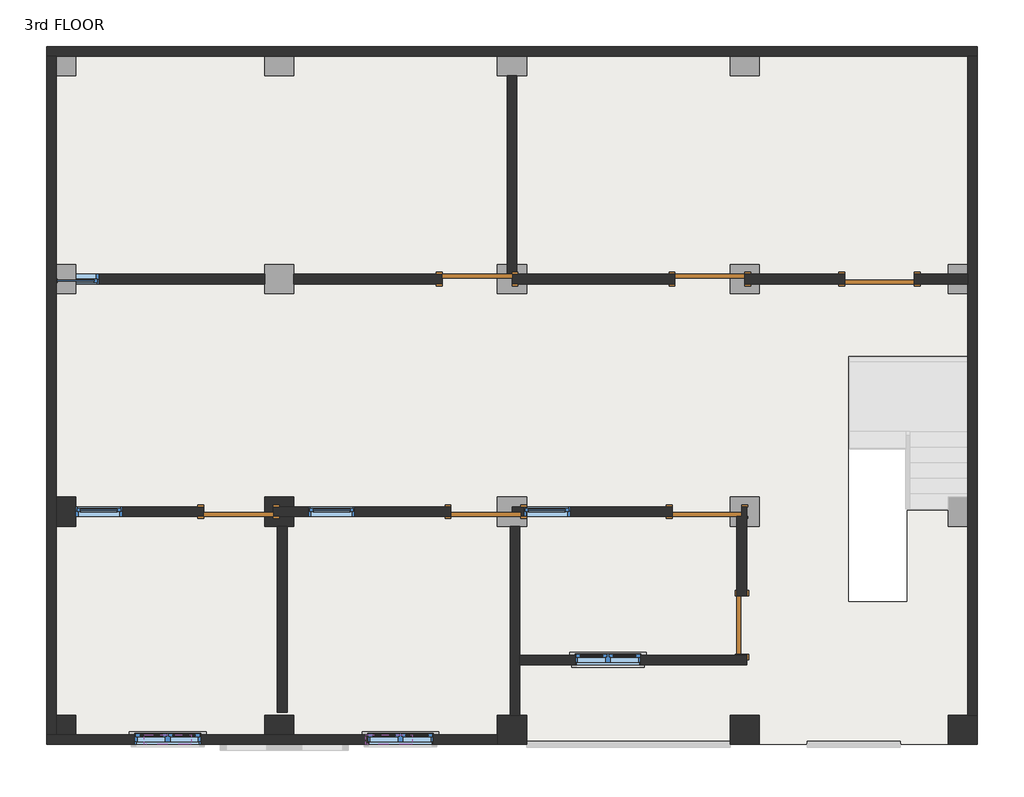
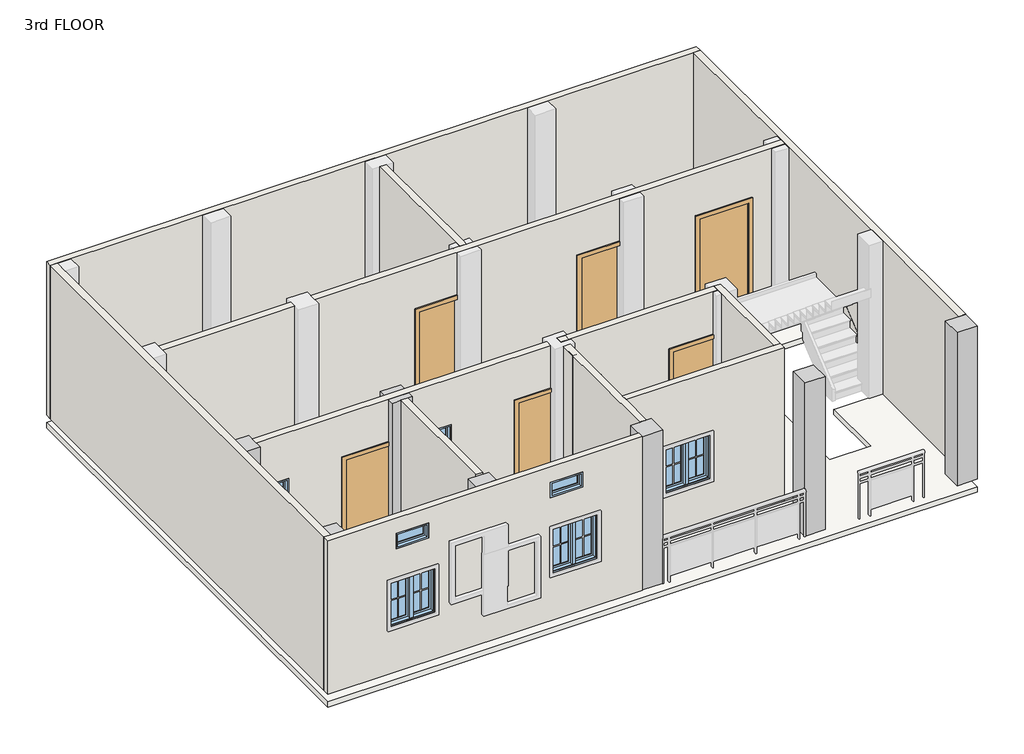
# One storey, part 1 of 2: 15 walls, 9 windows, 7 columns, 7 doors, 1 slab.
"""IFC4 building model written with IfcOpenShell, lengths in millimetres."""

from ifc_helpers import new_model, si_unit, frame, origin, place, context, project, spatial, polyline, outline, extrude, faceted_brep, transform, mapped, element, save
from components import door_e00f436c, door_a1797ceb, window_4c2727af, window_0bf3737e, window_78893e6c, window_0d9958e7

model = new_model("IFC4")

# Units and contexts
model_context = context("Model", 3, world=origin())
ifc_project = project(units=[si_unit("LENGTHUNIT", "METRE", prefix="MILLI")], contexts=[model_context])

# Site, building, storey
site = spatial("IfcSite", under=ifc_project)
building = spatial("IfcBuilding", under=site)
storey = spatial("IfcBuildingStorey", under=building, Name="3rd FLOOR", Elevation=8991.6)

# Columns
placement = place(None, origin())
element("IfcColumn", 1, ObjectType="column family : column family", at=placement, inside=storey, context=model_context, shape_type="Brep", body=[
    faceted_brep([(-12576.097125, 2486.2065522, 8996.6), (-12957.097125, 2486.2065522, 8996.6), (-12957.097125, 2867.2065522, 8996.6), (-12576.097125, 2867.2065522, 8996.6), (-12576.097125, 2740.2065522, 8996.6), (-12842.797125, 2740.2065522, 8996.6), (-12842.797125, 2613.2065522, 8996.6), (-12576.097125, 2613.2065522, 8996.6), (-12576.097125, 2486.2065522, 12034.6), (-12576.097125, 2613.2065522, 12034.6), (-12957.097125, 2486.2065522, 12034.6), (-12957.097125, 2613.2065522, 12034.6), (-12957.097125, 2613.2065522, 11125.2), (-12957.097125, 2740.2065522, 11125.2), (-12957.097125, 2740.2065522, 12034.6), (-12957.097125, 2867.2065522, 12034.6), (-12576.097125, 2867.2065522, 12034.6), (-12842.797125, 2613.2065522, 11125.2), (-12842.797125, 2740.2065522, 11125.2), (-12576.097125, 2740.2065522, 12034.6)], [[[0, 1, 2, 3, 4, 5, 6, 7]], [[8, 0, 7, 9]], [[1, 0, 8, 10]], [[2, 1, 10, 11, 12, 13, 14, 15]], [[3, 2, 15, 16]], [[10, 8, 9, 11]], [[6, 17, 12, 11, 9, 7]], [[13, 18, 5, 4, 19, 14]], [[3, 16, 19, 4]], [[16, 15, 14, 19]], [[17, 18, 13, 12]], [[18, 17, 6, 5]]]),
])
element("IfcColumn", 2, ObjectType="column family : column family", at=placement, inside=storey, context=model_context, shape_type="SweptSolid", body=[
    extrude(outline(polyline([(-15433.597125, 2867.2065522), (-15433.597125, 2486.2065522), (-15687.597125, 2486.2065522), (-15687.597125, 2867.2065522), (-15433.597125, 2867.2065522)])), frame((0.0, 0.0, 8996.6), z_axis=(0.0, 0.0, 1.0), x_axis=(1.0, 0.0, 0.0)), (0.0, 0.0, 1.0), 3038.0),
])
element("IfcColumn", 3, ObjectType="column family : column family", at=placement, inside=storey, context=model_context, shape_type="SweptSolid", body=[
    extrude(outline(polyline([(-15433.597125, 9.7065522), (-15433.597125, -244.2934478), (-15687.597125, -244.2934478), (-15687.597125, 9.7065522), (-15433.597125, 9.7065522)])), frame((0.0, 0.0, 8996.6), z_axis=(0.0, 0.0, 1.0), x_axis=(1.0, 0.0, 0.0)), (0.0, 0.0, 1.0), 3038.0),
])
element("IfcColumn", 4, ObjectType="column family : column family", at=placement, inside=storey, context=model_context, shape_type="SweptSolid", body=[
    extrude(outline(polyline([(-3622.597125, 9.7065522), (-3622.597125, -371.2934478), (-4003.597125, -371.2934478), (-4003.597125, 9.7065522), (-3622.597125, 9.7065522)])), frame((0.0, 0.0, 8996.6), z_axis=(0.0, 0.0, 1.0), x_axis=(1.0, 0.0, 0.0)), (0.0, 0.0, 1.0), 3038.0),
])
element("IfcColumn", 5, ObjectType="column family : column family", at=placement, inside=storey, context=model_context, shape_type="SweptSolid", body=[
    extrude(outline(polyline([(-6480.097125, 9.7065522), (-6480.097125, -371.2934478), (-6861.097125, -371.2934478), (-6861.097125, 9.7065522), (-6480.097125, 9.7065522)])), frame((0.0, 0.0, 8996.6), z_axis=(0.0, 0.0, 1.0), x_axis=(1.0, 0.0, 0.0)), (0.0, 0.0, 1.0), 3038.0),
])
element("IfcColumn", 6, ObjectType="column family : column family", at=placement, inside=storey, context=model_context, shape_type="SweptSolid", body=[
    extrude(outline(polyline([(-9528.097125, 9.7065522), (-9528.097125, -371.2934478), (-9909.097125, -371.2934478), (-9909.097125, 9.7065522), (-9528.097125, 9.7065522)])), frame((0.0, 0.0, 8996.6), z_axis=(0.0, 0.0, 1.0), x_axis=(1.0, 0.0, 0.0)), (0.0, 0.0, 1.0), 3038.0),
])
element("IfcColumn", 7, ObjectType="column family : column family", at=placement, inside=storey, context=model_context, shape_type="SweptSolid", body=[
    extrude(outline(polyline([(-12957.097125, 9.7065522), (-12576.097125, 9.7065522), (-12576.097125, -244.2934478), (-12957.097125, -244.2934478), (-12957.097125, 9.7065522)])), frame((0.0, 0.0, 8996.6), z_axis=(0.0, 0.0, 1.0), x_axis=(1.0, 0.0, 0.0)), (0.0, 0.0, 1.0), 3038.0),
])

# Doors
door_shape = door_e00f436c(model_context)
element("IfcDoor", 8, ObjectType="Single-Flush : 30\" x 80\"", at=placement, inside=storey, context=model_context, shape_type="MappedRepresentation", body=[
    mapped(door_shape, transform((-6708.697125, 1190.8065522, 8991.6), x_axis=(0.0, -1.0, 0.0), y_axis=(1.0, 0.0, 0.0), z_axis=(0.0, 0.0, 1.0))),
])
door_2_shape = door_a1797ceb(model_context)
element("IfcDoor", 9, ObjectType="Single-Flush : 36\" x 84\"", at=placement, inside=storey, context=model_context, shape_type="MappedRepresentation", body=[
    mapped(door_2_shape, transform((-10175.797125, 5724.7065522, 8991.6), x_axis=(1.0, 0.0, 0.0), y_axis=(0.0, 1.0, 0.0), z_axis=(0.0, 0.0, 1.0))),
])
element("IfcDoor", 10, ObjectType="Single-Flush : 36\" x 84\"", at=placement, inside=storey, context=model_context, shape_type="MappedRepresentation", body=[
    mapped(door_2_shape, transform((-10061.497125, 2676.7065522, 8991.6), x_axis=(-1.0, 0.0, 0.0), y_axis=(0.0, -1.0, 0.0), z_axis=(0.0, 0.0, 1.0))),
])
element("IfcDoor", 11, ObjectType="Single-Flush : 36\" x 84\"", at=placement, inside=storey, context=model_context, shape_type="MappedRepresentation", body=[
    mapped(door_2_shape, transform((-13299.997125, 2676.7065522, 8991.6), x_axis=(-1.0, 0.0, 0.0), y_axis=(0.0, -1.0, 0.0), z_axis=(0.0, 0.0, 1.0))),
])
element("IfcDoor", 12, ObjectType="Single-Flush : 36\" x 84\"", at=placement, inside=storey, context=model_context, shape_type="MappedRepresentation", body=[
    mapped(door_2_shape, transform((-7127.797125, 5724.7065522, 8991.6), x_axis=(1.0, 0.0, 0.0), y_axis=(0.0, 1.0, 0.0), z_axis=(0.0, 0.0, 1.0))),
])
element("IfcDoor", 13, ObjectType="Single-Flush : 36\" x 84\"", at=placement, inside=storey, context=model_context, shape_type="MappedRepresentation", body=[
    mapped(door_2_shape, transform((-7165.897125, 2676.7065522, 8991.6), x_axis=(-1.0, 0.0, 0.0), y_axis=(0.0, -1.0, 0.0), z_axis=(0.0, 0.0, 1.0))),
])
element("IfcDoor", 14, ObjectType="Single-Flush : 36\" x 84\"", at=placement, inside=storey, context=model_context, shape_type="MappedRepresentation", body=[
    mapped(door_2_shape, transform((-4905.297125, 5724.7065522, 8991.6), x_axis=(-1.0, 0.0, 0.0), y_axis=(0.0, -1.0, 0.0), z_axis=(0.0, 0.0, 1.0))),
])

# Slab
element("IfcSlab", 15, ObjectType="Generic - 4\"", at=placement, inside=storey, context=model_context, shape_type="SweptSolid", body=[
    extrude(outline(polyline([(-3622.597125, 8772.7065522), (-3622.597125, -371.2934478), (-15814.597125, -371.2934478), (-15814.597125, 8772.7065522), (-3622.597125, 8772.7065522)]), holes=[polyline([(-3734.357125, 4711.0719226), (-5310.2646464, 4711.0719226), (-5310.2646464, 1502.3126957), (-4547.7736682, 1502.3126957), (-4547.7736682, 2699.911213), (-3734.357125, 2699.911213), (-3734.357125, 4711.0719226)])]), frame((0.0, 0.0, 8737.6), z_axis=(0.0, 0.0, 1.0), x_axis=(1.0, 0.0, 0.0)), (0.0, 0.0, 1.0), 101.6),
])

# Walls
element("IfcWall", 16, ObjectType="Generic - 5\"", at=placement, inside=storey, context=model_context, shape_type="Brep", body=[
    faceted_brep([(-15814.597125, 8645.7065522, 8991.6), (-15687.597125, 8645.7065522, 8991.6), (-3749.597125, 8645.7065522, 8991.6), (-3622.597125, 8645.7065522, 8991.6), (-3622.597125, 8645.7065522, 12039.6), (-3749.597125, 8645.7065522, 12039.6), (-15687.597125, 8645.7065522, 12039.6), (-15814.597125, 8645.7065522, 12039.6), (-15814.597125, 8772.7065522, 8991.6), (-15814.597125, 8772.7065522, 12039.6), (-3622.597125, 8772.7065522, 12039.6), (-3622.597125, 8772.7065522, 8991.6)], [[[0, 1, 2, 3, 4, 5, 6, 7]], [[8, 9, 10, 11]], [[3, 2, 1, 0, 8, 11]], [[7, 6, 5, 4, 10, 9]], [[4, 3, 11, 10]], [[0, 7, 9, 8]]]),
])
element("IfcWall", 17, ObjectType="Generic - 5\"", at=placement, inside=storey, context=model_context, shape_type="Brep", body=[
    faceted_brep([(-3749.597125, 8645.7065522, 8991.6), (-3749.597125, 5788.2065522, 8991.6), (-3749.597125, 5661.2065522, 8991.6), (-3749.597125, 9.7065522, 8991.6), (-3749.597125, 9.7065522, 12039.6), (-3749.597125, 5661.2065522, 12039.6), (-3749.597125, 5788.2065522, 12039.6), (-3749.597125, 8645.7065522, 12039.6), (-3622.597125, 8645.7065522, 8991.6), (-3622.597125, 8645.7065522, 12039.6), (-3622.597125, 9.7065522, 12039.6), (-3622.597125, 9.7065522, 12034.6), (-3622.597125, 9.7065522, 8996.6), (-3622.597125, 9.7065522, 8991.6)], [[[0, 1, 2, 3, 4, 5, 6, 7]], [[8, 9, 10, 11, 12, 13]], [[3, 2, 1, 0, 8, 13]], [[4, 3, 13, 12, 11, 10]], [[7, 6, 5, 4, 10, 9]], [[0, 7, 9, 8]]]),
])
element("IfcWall", 18, ObjectType="Generic - 5\"", at=placement, inside=storey, context=model_context, shape_type="Brep", body=[
    faceted_brep([(-9909.097125, -244.2934478, 8991.6), (-15687.597125, -244.2934478, 8991.6), (-15814.597125, -244.2934478, 8991.6), (-15814.597125, -244.2934478, 12039.6), (-15687.597125, -244.2934478, 12039.6), (-9909.097125, -244.2934478, 12039.6), (-13795.297125, -244.2934478, 10820.4), (-14658.897125, -244.2934478, 10820.4), (-14658.897125, -244.2934478, 9906.0), (-13795.297125, -244.2934478, 9906.0), (-10747.297125, -244.2934478, 10820.4), (-11610.897125, -244.2934478, 10820.4), (-11610.897125, -244.2934478, 9906.0), (-10747.297125, -244.2934478, 9906.0), (-13922.297125, -244.2934478, 11734.8), (-14531.897125, -244.2934478, 11734.8), (-14531.897125, -244.2934478, 11430.0), (-13922.297125, -244.2934478, 11430.0), (-11026.697125, -244.2934478, 11734.8), (-11636.297125, -244.2934478, 11734.8), (-11636.297125, -244.2934478, 11430.0), (-11026.697125, -244.2934478, 11430.0), (-9909.097125, -371.2934478, 8991.6), (-9909.097125, -371.2934478, 8996.6), (-9909.097125, -371.2934478, 12034.6), (-9909.097125, -371.2934478, 12039.6), (-15814.597125, -371.2934478, 12039.6), (-15814.597125, -371.2934478, 8991.6), (-13795.297125, -371.2934478, 10820.4), (-13795.297125, -371.2934478, 9906.0), (-14658.897125, -371.2934478, 9906.0), (-14658.897125, -371.2934478, 10820.4), (-10747.297125, -371.2934478, 10820.4), (-10747.297125, -371.2934478, 9906.0), (-11610.897125, -371.2934478, 9906.0), (-11610.897125, -371.2934478, 10820.4), (-13922.297125, -371.2934478, 11734.8), (-13922.297125, -371.2934478, 11430.0), (-14531.897125, -371.2934478, 11430.0), (-14531.897125, -371.2934478, 11734.8), (-11026.697125, -371.2934478, 11734.8), (-11026.697125, -371.2934478, 11430.0), (-11636.297125, -371.2934478, 11430.0), (-11636.297125, -371.2934478, 11734.8)], [[[0, 1, 2, 3, 4, 5], [6, 7, 8, 9], [10, 11, 12, 13], [14, 15, 16, 17], [18, 19, 20, 21]], [[22, 23, 24, 25, 26, 27], [28, 29, 30, 31], [32, 33, 34, 35], [36, 37, 38, 39], [40, 41, 42, 43]], [[2, 1, 0, 22, 27]], [[5, 4, 3, 26, 25]], [[0, 5, 25, 24, 23, 22]], [[3, 2, 27, 26]], [[29, 28, 6, 9]], [[30, 29, 9, 8]], [[31, 30, 8, 7]], [[28, 31, 7, 6]], [[33, 32, 10, 13]], [[34, 33, 13, 12]], [[35, 34, 12, 11]], [[32, 35, 11, 10]], [[37, 36, 14, 17]], [[38, 37, 17, 16]], [[39, 38, 16, 15]], [[36, 39, 15, 14]], [[41, 40, 18, 21]], [[42, 41, 21, 20]], [[43, 42, 20, 19]], [[40, 43, 19, 18]]]),
])
element("IfcWall", 19, ObjectType="Generic - 5\"", at=placement, inside=storey, context=model_context, shape_type="Brep", body=[
    faceted_brep([(-15687.597125, -244.2934478, 8991.6), (-15687.597125, 8645.7065522, 8991.6), (-15687.597125, 8645.7065522, 8996.6), (-15687.597125, 8645.7065522, 12034.6), (-15687.597125, 8645.7065522, 12039.6), (-15687.597125, -244.2934478, 12039.6), (-15687.597125, -244.2934478, 12034.6), (-15687.597125, -244.2934478, 8996.6), (-15814.597125, -244.2934478, 8991.6), (-15814.597125, -244.2934478, 12039.6), (-15814.597125, 8645.7065522, 12039.6), (-15814.597125, 8645.7065522, 8991.6)], [[[0, 1, 2, 3, 4, 5, 6, 7]], [[8, 9, 10, 11]], [[1, 0, 8, 11]], [[5, 4, 10, 9]], [[4, 3, 2, 1, 11, 10]], [[0, 7, 6, 5, 9, 8]]]),
])
element("IfcWall", 20, ObjectType="Generic - 5\"", at=placement, inside=storey, context=model_context, shape_type="SweptSolid", body=[
    extrude(outline(polyline([(8991.6, -15433.597125), (8991.6, -12957.097125), (12039.6, -12957.097125), (12039.6, -15433.597125), (11125.2, -15433.597125), (11125.2, -15128.797125), (9296.4, -15128.797125), (9296.4, -15433.597125), (8991.6, -15433.597125)])), frame((0.0, 5661.2065522, 0.0), z_axis=(0.0, 1.0, 0.0), x_axis=(0.0, 0.0, 1.0)), (0.0, 0.0, 1.0), 127.0),
])
element("IfcWall", 21, ObjectType="Generic - 5\"", at=placement, inside=storey, context=model_context, shape_type="Brep", body=[
    faceted_brep([(-9782.097125, 8391.7065522, 8991.6), (-9782.097125, 5788.2065522, 8991.6), (-9782.097125, 5788.2065522, 8996.6), (-9782.097125, 5788.2065522, 11125.2), (-9782.097125, 5788.2065522, 12034.6), (-9782.097125, 5788.2065522, 12039.6), (-9782.097125, 8391.7065522, 12039.6), (-9655.097125, 8391.7065522, 8991.6), (-9655.097125, 8391.7065522, 12039.6), (-9655.097125, 5788.2065522, 12039.6), (-9655.097125, 5788.2065522, 12034.6), (-9655.097125, 5788.2065522, 8996.6), (-9655.097125, 5788.2065522, 8991.6), (-9718.597125, 5788.2065522, 8991.6)], [[[0, 1, 2, 3, 4, 5, 6]], [[7, 8, 9, 10, 11, 12]], [[1, 0, 7, 12, 13]], [[6, 5, 9, 8]], [[0, 6, 8, 7]], [[5, 4, 3, 2, 1, 13, 12, 11, 10, 9]]]),
])
element("IfcWall", 22, ObjectType="Generic - 5\"", at=placement, inside=storey, context=model_context, shape_type="Brep", body=[
    faceted_brep([(-6670.597125, 5661.2065522, 8991.6), (-5362.497125, 5661.2065522, 8991.6), (-5362.497125, 5661.2065522, 11125.2), (-4448.097125, 5661.2065522, 11125.2), (-4448.097125, 5661.2065522, 8991.6), (-3749.597125, 5661.2065522, 8991.6), (-3749.597125, 5661.2065522, 8996.6), (-3749.597125, 5661.2065522, 12034.6), (-3749.597125, 5661.2065522, 12039.6), (-12576.097125, 5661.2065522, 12039.6), (-12576.097125, 5661.2065522, 8991.6), (-10632.997125, 5661.2065522, 8991.6), (-10632.997125, 5661.2065522, 11125.2), (-9909.097125, 5661.2065522, 11125.2), (-9718.597125, 5661.2065522, 11125.2), (-9718.597125, 5661.2065522, 8996.6), (-9718.597125, 5661.2065522, 8991.6), (-7584.997125, 5661.2065522, 8991.6), (-7584.997125, 5661.2065522, 11125.2), (-6861.097125, 5661.2065522, 11125.2), (-6670.597125, 5661.2065522, 11125.2), (-6670.597125, 5661.2065522, 8996.6), (-5362.497125, 5788.2065522, 11125.2), (-5362.497125, 5788.2065522, 8991.6), (-6670.597125, 5788.2065522, 8991.6), (-6670.597125, 5788.2065522, 8996.6), (-6670.597125, 5788.2065522, 11125.2), (-6861.097125, 5788.2065522, 11125.2), (-7584.997125, 5788.2065522, 11125.2), (-7584.997125, 5788.2065522, 8991.6), (-9655.097125, 5788.2065522, 8991.6), (-9718.597125, 5788.2065522, 8991.6), (-9718.597125, 5788.2065522, 8996.6), (-9718.597125, 5788.2065522, 11125.2), (-9782.097125, 5788.2065522, 11125.2), (-9909.097125, 5788.2065522, 11125.2), (-10632.997125, 5788.2065522, 11125.2), (-10632.997125, 5788.2065522, 8991.6), (-12576.097125, 5788.2065522, 8991.6), (-12576.097125, 5788.2065522, 12039.6), (-9782.097125, 5788.2065522, 12039.6), (-9655.097125, 5788.2065522, 12039.6), (-3749.597125, 5788.2065522, 12039.6), (-3749.597125, 5788.2065522, 12034.6), (-3749.597125, 5788.2065522, 8996.6), (-3749.597125, 5788.2065522, 8991.6), (-4448.097125, 5788.2065522, 8991.6), (-4448.097125, 5788.2065522, 11125.2)], [[[0, 1, 2, 3, 4, 5, 6, 7, 8, 9, 10, 11, 12, 13, 14, 15, 16, 17, 18, 19, 20, 21]], [[22, 23, 24, 25, 26, 27, 28, 29, 30, 31, 32, 33, 34, 35, 36, 37, 38, 39, 40, 41, 42, 43, 44, 45, 46, 47]], [[11, 10, 38, 37]], [[17, 16, 31, 30, 29]], [[46, 45, 5, 4]], [[24, 23, 1, 0]], [[9, 8, 42, 41, 40, 39]], [[10, 9, 39, 38]], [[8, 7, 6, 5, 45, 44, 43, 42]], [[33, 32, 31, 16, 15, 14]], [[36, 35, 34, 33, 14, 13, 12]], [[37, 36, 12, 11]], [[26, 25, 24, 0, 21, 20]], [[28, 27, 26, 20, 19, 18]], [[29, 28, 18, 17]], [[2, 1, 23, 22]], [[3, 2, 22, 47]], [[4, 3, 47, 46]]]),
])
element("IfcWall", 23, ObjectType="Generic - 5\"", at=placement, inside=storey, context=model_context, shape_type="Brep", body=[
    faceted_brep([(-14823.997125, 2613.2065522, 9296.4), (-15433.597125, 2613.2065522, 9296.4), (-15433.597125, 2613.2065522, 8991.6), (-13757.197125, 2613.2065522, 8991.6), (-13757.197125, 2613.2065522, 11125.2), (-12957.097125, 2613.2065522, 11125.2), (-12842.797125, 2613.2065522, 11125.2), (-12842.797125, 2613.2065522, 8996.6), (-12842.797125, 2613.2065522, 8991.6), (-10518.697125, 2613.2065522, 8991.6), (-10518.697125, 2613.2065522, 11125.2), (-9909.097125, 2613.2065522, 11125.2), (-9909.097125, 2613.2065522, 12039.6), (-15433.597125, 2613.2065522, 12039.6), (-15433.597125, 2613.2065522, 11125.2), (-14823.997125, 2613.2065522, 11125.2), (-12385.597125, 2613.2065522, 11125.2), (-11775.997125, 2613.2065522, 11125.2), (-11775.997125, 2613.2065522, 9296.4), (-12385.597125, 2613.2065522, 9296.4), (-15433.597125, 2740.2065522, 8991.6), (-15433.597125, 2740.2065522, 9296.4), (-14823.997125, 2740.2065522, 9296.4), (-14823.997125, 2740.2065522, 11125.2), (-15433.597125, 2740.2065522, 11125.2), (-15433.597125, 2740.2065522, 12039.6), (-9909.097125, 2740.2065522, 12039.6), (-9909.097125, 2740.2065522, 11125.2), (-10518.697125, 2740.2065522, 11125.2), (-10518.697125, 2740.2065522, 8991.6), (-12842.797125, 2740.2065522, 8991.6), (-12842.797125, 2740.2065522, 8996.6), (-12842.797125, 2740.2065522, 11125.2), (-12957.097125, 2740.2065522, 11125.2), (-13757.197125, 2740.2065522, 11125.2), (-13757.197125, 2740.2065522, 8991.6), (-12385.597125, 2740.2065522, 11125.2), (-12385.597125, 2740.2065522, 9296.4), (-11775.997125, 2740.2065522, 9296.4), (-11775.997125, 2740.2065522, 11125.2)], [[[0, 1, 2, 3, 4, 5, 6, 7, 8, 9, 10, 11, 12, 13, 14, 15], [16, 17, 18, 19]], [[20, 21, 22, 23, 24, 25, 26, 27, 28, 29, 30, 31, 32, 33, 34, 35], [36, 37, 38, 39]], [[30, 29, 9, 8]], [[20, 35, 3, 2]], [[26, 12, 11, 27]], [[13, 12, 26, 25]], [[14, 13, 25, 24]], [[2, 1, 21, 20]], [[28, 10, 9, 29]], [[10, 28, 27, 11]], [[4, 3, 35, 34]], [[6, 5, 4, 34, 33, 32]], [[8, 7, 6, 32, 31, 30]], [[22, 21, 1, 0]], [[23, 22, 0, 15]], [[24, 23, 15, 14]], [[37, 36, 16, 19]], [[38, 37, 19, 18]], [[39, 38, 18, 17]], [[36, 39, 17, 16]]]),
])
element("IfcWall", 24, ObjectType="Generic - 5\"", at=placement, inside=storey, context=model_context, shape_type="Brep", body=[
    faceted_brep([(-9616.997125, 9.7065522, 8991.6), (-9616.997125, 670.1065522, 8991.6), (-9616.997125, 797.1065522, 8991.6), (-9616.997125, 2486.2065522, 8991.6), (-9616.997125, 2486.2065522, 12039.6), (-9616.997125, 797.1065522, 12039.6), (-9616.997125, 670.1065522, 12039.6), (-9616.997125, 9.7065522, 12039.6), (-9743.997125, 9.7065522, 8991.6), (-9743.997125, 9.7065522, 12039.6), (-9743.997125, 2486.2065522, 12039.6), (-9743.997125, 2486.2065522, 8991.6)], [[[0, 1, 2, 3, 4, 5, 6, 7]], [[8, 9, 10, 11]], [[3, 2, 1, 0, 8, 11]], [[4, 3, 11, 10]], [[7, 6, 5, 4, 10, 9]], [[0, 7, 9, 8]]]),
])
element("IfcWall", 25, ObjectType="Generic - 5\"", at=placement, inside=storey, context=model_context, shape_type="SweptSolid", body=[
    extrude(outline(polyline([(-9743.997125, 2181.4065522), (-9743.997125, 2486.2065522), (-9616.997125, 2486.2065522), (-9616.997125, 2181.4065522), (-9743.997125, 2181.4065522)])), frame((0.0, 0.0, 8991.6), z_axis=(0.0, 0.0, 1.0), x_axis=(1.0, 0.0, 0.0)), (0.0, 0.0, 1.0), 3048.0),
])
element("IfcWall", 26, ObjectType="Generic - 5\"", at=placement, inside=storey, context=model_context, shape_type="Brep", body=[
    faceted_brep([(-6772.197125, 2613.2065522, 12039.6), (-9718.597125, 2613.2065522, 12039.6), (-9718.597125, 2613.2065522, 12034.6), (-9718.597125, 2613.2065522, 8996.6), (-9718.597125, 2613.2065522, 8991.6), (-7623.097125, 2613.2065522, 8991.6), (-7623.097125, 2613.2065522, 11125.2), (-6861.097125, 2613.2065522, 11125.2), (-6772.197125, 2613.2065522, 11125.2), (-6772.197125, 2613.2065522, 12034.6), (-9566.197125, 2613.2065522, 11125.2), (-9528.097125, 2613.2065522, 11125.2), (-8956.597125, 2613.2065522, 11125.2), (-8956.597125, 2613.2065522, 9296.4), (-9528.097125, 2613.2065522, 9296.4), (-9566.197125, 2613.2065522, 9296.4), (-9718.597125, 2740.2065522, 12039.6), (-6772.197125, 2740.2065522, 12039.6), (-6772.197125, 2740.2065522, 11125.2), (-6861.097125, 2740.2065522, 11125.2), (-7623.097125, 2740.2065522, 11125.2), (-7623.097125, 2740.2065522, 8991.6), (-9718.597125, 2740.2065522, 8991.6), (-9718.597125, 2740.2065522, 8996.6), (-9718.597125, 2740.2065522, 12034.6), (-9566.197125, 2740.2065522, 11125.2), (-9566.197125, 2740.2065522, 9296.4), (-9528.097125, 2740.2065522, 9296.4), (-8956.597125, 2740.2065522, 9296.4), (-8956.597125, 2740.2065522, 11125.2), (-9528.097125, 2740.2065522, 11125.2)], [[[0, 1, 2, 3, 4, 5, 6, 7, 8, 9], [10, 11, 12, 13, 14, 15]], [[16, 17, 18, 19, 20, 21, 22, 23, 24], [25, 26, 27, 28, 29, 30]], [[4, 22, 21, 5]], [[1, 0, 17, 16]], [[4, 3, 2, 1, 16, 24, 23, 22]], [[26, 25, 10, 15]], [[28, 27, 26, 15, 14, 13]], [[29, 28, 13, 12]], [[25, 30, 29, 12, 11, 10]], [[20, 6, 5, 21]], [[6, 20, 19, 18, 8, 7]], [[17, 0, 9, 8, 18]]]),
])
element("IfcWall", 27, ObjectType="Generic - 5\"", at=placement, inside=storey, context=model_context, shape_type="Brep", body=[
    faceted_brep([(-6645.197125, 797.1065522, 8991.6), (-6645.197125, 809.8065522, 8991.6), (-6645.197125, 809.8065522, 11023.6), (-6645.197125, 1571.8065522, 11023.6), (-6645.197125, 1571.8065522, 8991.6), (-6645.197125, 2740.2065522, 8991.6), (-6645.197125, 2740.2065522, 8996.6), (-6645.197125, 2740.2065522, 12034.6), (-6645.197125, 2740.2065522, 12039.6), (-6645.197125, 797.1065522, 12039.6), (-6772.197125, 809.8065522, 11023.6), (-6772.197125, 809.8065522, 8991.6), (-6772.197125, 797.1065522, 8991.6), (-6772.197125, 797.1065522, 12039.6), (-6772.197125, 2613.2065522, 12039.6), (-6772.197125, 2740.2065522, 12039.6), (-6772.197125, 2740.2065522, 11125.2), (-6772.197125, 2613.2065522, 11125.2), (-6772.197125, 2613.2065522, 8996.6), (-6772.197125, 2613.2065522, 8991.6), (-6772.197125, 1571.8065522, 8991.6), (-6772.197125, 1571.8065522, 11023.6), (-6708.697125, 2613.2065522, 8991.6), (-6708.697125, 2740.2065522, 8991.6), (-6708.697125, 2613.2065522, 11125.2), (-6708.697125, 2613.2065522, 8996.6), (-6708.697125, 2740.2065522, 11125.2), (-6708.697125, 2740.2065522, 8996.6)], [[[0, 1, 2, 3, 4, 5, 6, 7, 8, 9]], [[10, 11, 12, 13, 14, 15, 16, 17, 18, 19, 20, 21]], [[20, 19, 22, 23, 5, 4]], [[12, 11, 1, 0]], [[9, 8, 15, 14, 13]], [[24, 25, 22, 19, 18, 17]], [[26, 24, 17, 16]], [[22, 25, 24, 26, 27, 23]], [[8, 7, 6, 5, 23, 27, 26, 16, 15]], [[0, 9, 13, 12]], [[2, 1, 11, 10]], [[3, 2, 10, 21]], [[4, 3, 21, 20]]]),
])
element("IfcWall", 28, ObjectType="Generic - 5\"", at=placement, inside=storey, context=model_context, shape_type="Brep", body=[
    faceted_brep([(-9718.597125, 2613.2065522, 8991.6), (-9566.197125, 2613.2065522, 8991.6), (-9566.197125, 2613.2065522, 9296.4), (-9566.197125, 2613.2065522, 11125.2), (-9566.197125, 2613.2065522, 12039.6), (-9718.597125, 2613.2065522, 12039.6), (-9718.597125, 2613.2065522, 12034.6), (-9718.597125, 2613.2065522, 8996.6), (-9718.597125, 2740.2065522, 8991.6), (-9718.597125, 2740.2065522, 8996.6), (-9718.597125, 2740.2065522, 12034.6), (-9718.597125, 2740.2065522, 12039.6), (-9566.197125, 2740.2065522, 12039.6), (-9566.197125, 2740.2065522, 11125.2), (-9566.197125, 2740.2065522, 9296.4), (-9566.197125, 2740.2065522, 8991.6)], [[[0, 1, 2, 3, 4, 5, 6, 7]], [[8, 9, 10, 11, 12, 13, 14, 15]], [[1, 0, 8, 15]], [[4, 3, 2, 1, 15, 14, 13, 12]], [[5, 4, 12, 11]], [[0, 7, 6, 5, 11, 10, 9, 8]]]),
])
element("IfcWall", 29, ObjectType="Generic - 5\"", at=placement, inside=storey, context=model_context, shape_type="SweptSolid", body=[
    extrude(outline(polyline([(-12791.997125, 47.8065522), (-12791.997125, 2486.2065522), (-12664.997125, 2486.2065522), (-12664.997125, 47.8065522), (-12791.997125, 47.8065522)])), frame((0.0, 0.0, 8991.6), z_axis=(0.0, 0.0, 1.0), x_axis=(1.0, 0.0, 0.0)), (0.0, 0.0, 1.0), 3048.0),
])
element("IfcWall", 30, ObjectType="Generic - 5\"", at=placement, inside=storey, context=model_context, shape_type="Brep", body=[
    faceted_brep([(-9616.997125, 670.1065522, 8991.6), (-6645.197125, 670.1065522, 8991.6), (-6645.197125, 670.1065522, 12039.6), (-9616.997125, 670.1065522, 12039.6), (-8029.497125, 670.1065522, 10820.4), (-8029.497125, 670.1065522, 9906.0), (-8893.097125, 670.1065522, 9906.0), (-8893.097125, 670.1065522, 10820.4), (-9616.997125, 797.1065522, 8991.6), (-9616.997125, 797.1065522, 12039.6), (-6772.197125, 797.1065522, 12039.6), (-6645.197125, 797.1065522, 12039.6), (-6645.197125, 797.1065522, 8991.6), (-6772.197125, 797.1065522, 8991.6), (-8029.497125, 797.1065522, 10820.4), (-8893.097125, 797.1065522, 10820.4), (-8893.097125, 797.1065522, 9906.0), (-8029.497125, 797.1065522, 9906.0)], [[[0, 1, 2, 3], [4, 5, 6, 7]], [[8, 9, 10, 11, 12, 13], [14, 15, 16, 17]], [[1, 0, 8, 13, 12]], [[3, 2, 11, 10, 9]], [[0, 3, 9, 8]], [[2, 1, 12, 11]], [[5, 4, 14, 17]], [[6, 5, 17, 16]], [[7, 6, 16, 15]], [[4, 7, 15, 14]]]),
])

# Windows
window_shape = window_4c2727af(model_context)
element("IfcWindow", 31, ObjectType="Fixed : 24\" x 12\"", at=placement, inside=storey, context=model_context, shape_type="MappedRepresentation", body=[
    mapped(window_shape, transform((-14188.997125, -307.7934478, 10515.6), x_axis=(1.0, 0.0, 0.0), y_axis=(0.0, 1.0, 0.0), z_axis=(0.0, 0.0, 1.0))),
])
element("IfcWindow", 32, ObjectType="Fixed : 24\" x 12\"", at=placement, inside=storey, context=model_context, shape_type="MappedRepresentation", body=[
    mapped(window_shape, transform((-11293.397125, -307.7934478, 10515.6), x_axis=(1.0, 0.0, 0.0), y_axis=(0.0, 1.0, 0.0), z_axis=(0.0, 0.0, 1.0))),
])
window_2_shape = window_0bf3737e(model_context)
element("IfcWindow", 33, ObjectType="Fixed : 24\" x 72\"", at=placement, inside=storey, context=model_context, shape_type="MappedRepresentation", body=[
    mapped(window_2_shape, transform((-15471.697125, 5724.7065522, 8991.6), x_axis=(-1.0, 0.0, 0.0), y_axis=(0.0, -1.0, 0.0), z_axis=(0.0, 0.0, 1.0))),
])
window_3_shape = window_78893e6c(model_context)
element("IfcWindow", 34, ObjectType="Fixed : 24\" x 72\"", at=placement, inside=storey, context=model_context, shape_type="MappedRepresentation", body=[
    mapped(window_3_shape, transform((-15166.897125, 2676.7065522, 8991.6), x_axis=(-1.0, 0.0, 0.0), y_axis=(0.0, -1.0, 0.0), z_axis=(0.0, 0.0, 1.0))),
])
element("IfcWindow", 35, ObjectType="Fixed : 24\" x 72\"", at=placement, inside=storey, context=model_context, shape_type="MappedRepresentation", body=[
    mapped(window_3_shape, transform((-12118.897125, 2676.7065522, 8991.6), x_axis=(-1.0, 0.0, 0.0), y_axis=(0.0, -1.0, 0.0), z_axis=(0.0, 0.0, 1.0))),
])
element("IfcWindow", 36, ObjectType="Fixed : 24\" x 72\"", at=placement, inside=storey, context=model_context, shape_type="MappedRepresentation", body=[
    mapped(window_3_shape, transform((-9299.497125, 2676.7065522, 8991.6), x_axis=(-1.0, 0.0, 0.0), y_axis=(0.0, -1.0, 0.0), z_axis=(0.0, 0.0, 1.0))),
])
window_4_shape = window_0d9958e7(model_context)
element("IfcWindow", 37, ObjectType="Window-Casement-Double : 34\" x 36\"", at=placement, inside=storey, context=model_context, shape_type="MappedRepresentation", body=[
    mapped(window_4_shape, transform((-14227.097125, -307.7934478, 8991.6), x_axis=(1.0, 0.0, 0.0), y_axis=(0.0, 1.0, 0.0), z_axis=(0.0, 0.0, 1.0))),
])
element("IfcWindow", 38, ObjectType="Window-Casement-Double : 34\" x 36\"", at=placement, inside=storey, context=model_context, shape_type="MappedRepresentation", body=[
    mapped(window_4_shape, transform((-11179.097125, -307.7934478, 8991.6), x_axis=(1.0, 0.0, 0.0), y_axis=(0.0, 1.0, 0.0), z_axis=(0.0, 0.0, 1.0))),
])
element("IfcWindow", 39, ObjectType="Window-Casement-Double : 34\" x 36\"", at=placement, inside=storey, context=model_context, shape_type="MappedRepresentation", body=[
    mapped(window_4_shape, transform((-8461.297125, 733.6065522, 8991.6), x_axis=(1.0, 0.0, 0.0), y_axis=(0.0, 1.0, 0.0), z_axis=(0.0, 0.0, 1.0))),
])

save(model, "model.ifc")

# Revit data of these elements
# Type "column family : column family"
#   w2 [instance default] = 0' - 9.88189"
#   w1 [instance default] = 0' - 9.01575"
#   Depth = 1' - 11.62205"
#   Width = 1' - 11.62205"
# Type "Single-Flush : 30\" x 80\""
#   Type Mark = "5"
#   Construction Type Id = "MDOOR"
#   Assembly Code = "C1020"
#   Analytic Construction = "Metal"
#   Thickness = 0' - 2"
#   Heat Transfer Coefficient (U) = 0.651978 BTU/(h·ft²·°F)
#   Height = 6' - 8"
#   Trim Projection Ext = 0' - 1"
#   Trim Projection Int = 0' - 1"
#   Trim Width = 0' - 3"
#   Width = 2' - 6"
#   Define Thermal Properties by = 1
#   Define Thermal Properties by = 1
#   Door Material = Door - Panel
#   Frame Material = Door - Frame
#   Visual Light Transmittance = 0
#   Solar Heat Gain Coefficient = 0
#   Function = (empty or 0)
#   Wall Closure = (empty or 0)
# Type "Single-Flush : 36\" x 84\""
#   Type Mark = "1"
#   Construction Type Id = "MDOOR"
#   Assembly Code = "C1020"
#   Analytic Construction = "Metal"
#   Thickness = 0' - 2"
#   Heat Transfer Coefficient (U) = 0.651978 BTU/(h·ft²·°F)
#   Height = 7' - 0"
#   Trim Projection Ext = 0' - 1"
#   Trim Projection Int = 0' - 1"
#   Trim Width = 0' - 3"
#   Width = 3' - 0"
#   Define Thermal Properties by = 1
#   Define Thermal Properties by = 1
#   Door Material = Door - Panel
#   Frame Material = Door - Frame
#   Visual Light Transmittance = 0
#   Solar Heat Gain Coefficient = 0
#   Function = (empty or 0)
#   Wall Closure = (empty or 0)
# Type "Generic - 4\""
#   Assembly Code = "B1010"
#   Function = 0
#   Layers, outside or top first: 0' - 4" no material (function 1)
# Type "Generic - 5\""
#   Assembly Code = "B2010"
#   Layers, outside or top first: 0' - 5" no material (function 1)
# Type "Fixed : 24\" x 12\""
#   Type Mark = "4"
#   Construction Type Id = "GSP4R"
#   Assembly Code = "B2020100"
#   Analytic Construction = "1/8 in Pilkington single glazing"
#   Visual Light Transmittance = 0.9
#   Solar Heat Gain Coefficient = 0.78
#   Heat Transfer Coefficient (U) = 0.6496 BTU/(h·ft²·°F)
#   Height = 1' - 0"
#   Default Sill Height = 3' - 0"
#   Width = 2' - 0"
#   Window Inset = 0' - 0 3/4"
#   Define Thermal Properties by = 1
#   Define Thermal Properties by = 1
#   Glass Pane Material = Glass
#   Sash Material = Sash
#   Wall Closure = (empty or 0)
# Type "Fixed : 24\" x 72\""
#   Type Mark = "7"
#   Construction Type Id = "GSP4R"
#   Assembly Code = "B2020100"
#   Analytic Construction = "1/8 in Pilkington single glazing"
#   Visual Light Transmittance = 0.9
#   Solar Heat Gain Coefficient = 0.78
#   Heat Transfer Coefficient (U) = 0.6496 BTU/(h·ft²·°F)
#   Height = 6' - 0"
#   Default Sill Height = 1' - 0"
#   Width = 2' - 0"
#   Window Inset = 0' - 0 3/4"
#   Define Thermal Properties by = 1
#   Define Thermal Properties by = 1
#   Glass Pane Material = Glass
#   Sash Material = Sash
#   Wall Closure = (empty or 0)
# Type "Window-Casement-Double : 34\" x 36\""
#   Type Mark = "14"
#   Fire Rating = "0.5h"
#   Assembly Code = "B2020100"
#   Analytic Construction = "Double glazing - domestic"
#   Frame Extension [instance default] = 0' - 0 1/4"
#   Window Inset [instance default] = 0' - 0"
#   Wall Thickness [instance default] = 0' - 6"
#   Interior Wall Closure [instance default] = 0' - 2 1/4"
#   Half Width = 1' - 5"
#   Visual Light Transmittance = 0.81
#   Thermal Resistance (R) = 1.8146 (h·ft²·°F)/BTU
#   Solar Heat Gain Coefficient = 0.76
#   Rough Width = 2' - 10 1/2"
#   Rough Height = 3' - 0 1/2"
#   Height = 3' - 0"
#   Heat Transfer Coefficient (U) = 0.5511 BTU/(h·ft²·°F)
#   Exterior Wall Closure [instance default] = 0' - 1 1/4"
#   Extension Jamb [instance default] = 0' - 2 1/4"
#   Default Sill Height = 3' - 0"
#   Width = 2' - 10"
#   Define Thermal Properties by = 0
#   Muntin Visibility = yes
#   Interior Trim Visibility [instance default] = yes
#   Exterior Trim Visibility [instance default] = yes
#   Extension Jamb Visibility [instance default] = yes
#   Interior Trim Material = Wood - Stained
#   Muntin Pattern = Muntin Pattern_2x2 : Muntin Pattern_2x2
#   Interior Trim = Trim-Window-Interior-Flat : Picture Frame
#   Interior Frame Material = Wood - Stained
#   Glass Panel Material = Glass
#   Exterior Trim Material = Clad - White
#   Exterior Trim = Trim-Window-Exterior-Flat : with Sill
#   Exterior Frame Material = Clad - White
#   Wall Closure = (empty or 0)
# Element 1 (IfcColumn, "column family : column family")
#   w2 = 1' - 3"
#   w1 = 1' - 3"
#   Phase Created = New Construction
#   Materials on its faces: "Default Wall", "inside wall"
# Element 2 (IfcColumn, "column family : column family")
#   w2 = 1' - 3"
#   w1 = 0' - 10"
#   Phase Created = New Construction
#   Materials on its faces: "inside wall", "Default Wall"
# Elements 3, 7 (IfcColumn, "column family : column family")
#   w2 = 1' - 3"
#   w1 = 1' - 3"
#   Phase Created = New Construction
#   Materials on its faces: "Default Wall"
# Element 4 (IfcColumn, "column family : column family")
#   w2 = 1' - 3"
#   w1 = 1' - 3"
#   Phase Created = New Construction
#   Materials on its faces: "Clad - White", "Default Wall"
# Element 5 (IfcColumn, "column family : column family")
#   w2 = 1' - 3"
#   w1 = 1' - 3"
#   Phase Created = New Construction
#   Materials on its faces: "out side wall"
# Element 6 (IfcColumn, "column family : column family")
#   w2 = 1' - 3"
#   w1 = 1' - 3"
#   Phase Created = New Construction
#   Materials on its faces: "out side wall", "Default Wall"
# Element 8 (IfcDoor, "Single-Flush : 30\" x 80\"")
#   Phase Created = New Construction
#   Materials on its faces: "Door - Frame", "Door - Panel"
# Elements 9, 10, 11, 12, 13, 14 (IfcDoor, "Single-Flush : 36\" x 84\"")
#   Phase Created = New Construction
#   Materials on its faces: "Door - Frame", "Door - Panel"
# Element 15 (IfcSlab, "Generic - 4\"")
#   Height Offset From Level = -0' - 6"
#   Phase Created = New Construction
#   Materials on its faces: "Default Floor", "Clad - White", "floor"
# Element 16 (IfcWall, "Generic - 5\"")
#   Top Offset = 0' - 0"
#   Base Offset = 0' - 0"
#   wall height = 10' - 0"
#   Phase Created = New Construction
#   Base Constraint = 3rd FLOOR
#   Top Constraint = 4th FLOOR
#   Materials on its faces: "Default Wall", "Clad - White"
# Element 17 (IfcWall, "Generic - 5\"")
#   Top Offset = 0' - 0"
#   Base Offset = 0' - 0"
#   wall height = 10' - 0"
#   Phase Created = New Construction
#   Base Constraint = 3rd FLOOR
#   Top Constraint = 4th FLOOR
#   Materials on its faces: "Default Wall", "grey", "Clad - White"
# Element 18 (IfcWall, "Generic - 5\"")
#   Top Offset = 0' - 0"
#   Base Offset = 0' - 0"
#   wall height = 10' - 0"
#   Phase Created = New Construction
#   Base Constraint = 3rd FLOOR
#   Top Constraint = 4th FLOOR
#   Materials on its faces: "Default Wall", "out side wall", "Clad - White"
# Element 19 (IfcWall, "Generic - 5\"")
#   Top Offset = 0' - 0"
#   Base Offset = 0' - 0"
#   wall height = 10' - 0"
#   Phase Created = New Construction
#   Base Constraint = 3rd FLOOR
#   Top Constraint = 4th FLOOR
#   Materials on its faces: "Default Wall", "inside wall", "Clad - White"
# Elements 20, 23, 26, 27 (IfcWall, "Generic - 5\"")
#   Top Offset = 0' - 0"
#   Base Offset = 0' - 0"
#   wall height = 10' - 0"
#   Phase Created = New Construction
#   Base Constraint = 3rd FLOOR
#   Top Constraint = 4th FLOOR
#   Materials on its faces: "Default Wall", "inside wall"
# Elements 21, 25, 28, 29 (IfcWall, "Generic - 5\"")
#   Top Offset = 0' - 0"
#   Base Offset = 0' - 0"
#   wall height = 10' - 0"
#   Phase Created = New Construction
#   Base Constraint = 3rd FLOOR
#   Top Constraint = 4th FLOOR
#   Materials on its faces: "Default Wall"
# Elements 22, 24 (IfcWall, "Generic - 5\"")
#   Top Offset = 0' - 0"
#   Base Offset = 0' - 0"
#   wall height = 10' - 0"
#   Phase Created = New Construction
#   Base Constraint = 3rd FLOOR
#   Top Constraint = 4th FLOOR
#   Materials on its faces: "Default Wall", "grey"
# Element 30 (IfcWall, "Generic - 5\"")
#   Top Offset = 0' - 0"
#   Base Offset = 0' - 0"
#   wall height = 10' - 0"
#   Phase Created = New Construction
#   Base Constraint = 3rd FLOOR
#   Top Constraint = 4th FLOOR
#   Materials on its faces: "Default Wall", "grey", "inside wall"
# Element 31 (IfcWindow, "Fixed : 24\" x 12\"")
#   Mark = "34"
#   Phase Created = New Construction
#   Materials on its faces: "Sash", "Glass"
# Element 32 (IfcWindow, "Fixed : 24\" x 12\"")
#   Mark = "35"
#   Phase Created = New Construction
#   Materials on its faces: "Sash", "Glass"
# Element 33 (IfcWindow, "Fixed : 24\" x 72\"")
#   Mark = "28"
#   Phase Created = New Construction
#   Materials on its faces: "Sash", "Glass"
# Element 34 (IfcWindow, "Fixed : 24\" x 72\"")
#   Mark = "29"
#   Phase Created = New Construction
#   Materials on its faces: "Sash", "Glass"
# Element 35 (IfcWindow, "Fixed : 24\" x 72\"")
#   Mark = "30"
#   Phase Created = New Construction
#   Materials on its faces: "Sash", "Glass"
# Element 36 (IfcWindow, "Fixed : 24\" x 72\"")
#   Mark = "31"
#   Phase Created = New Construction
#   Materials on its faces: "Sash", "Glass"
# Element 37 (IfcWindow, "Window-Casement-Double : 34\" x 36\"")
#   Mark = "32"
#   Window Inset = 0' - 0"
#   Interior Wall Closure = 0' - 2 1/4"
#   Frame Extension = 0' - 0 1/4"
#   Exterior Wall Closure = 0' - 1 1/4"
#   Interior Trim Visibility = yes
#   Exterior Trim Visibility = yes
#   Phase Created = New Construction
#   Materials on its faces: "Wood - Stained", "Glass", "Clad - White"
# Element 38 (IfcWindow, "Window-Casement-Double : 34\" x 36\"")
#   Mark = "33"
#   Window Inset = 0' - 0"
#   Interior Wall Closure = 0' - 2 1/4"
#   Frame Extension = 0' - 0 1/4"
#   Exterior Wall Closure = 0' - 1 1/4"
#   Interior Trim Visibility = yes
#   Exterior Trim Visibility = yes
#   Phase Created = New Construction
#   Materials on its faces: "Wood - Stained", "Glass", "Clad - White"
# Element 39 (IfcWindow, "Window-Casement-Double : 34\" x 36\"")
#   Mark = "36"
#   Window Inset = 0' - 0"
#   Interior Wall Closure = 0' - 2 1/4"
#   Frame Extension = 0' - 0 1/4"
#   Exterior Wall Closure = 0' - 1 1/4"
#   Interior Trim Visibility = yes
#   Exterior Trim Visibility = yes
#   Phase Created = New Construction
#   Materials on its faces: "Wood - Stained", "Glass", "Clad - White"
# Materials
#   "Door - Panel": class "Wood", colour RGB 210 159 95, transparency 0, Cost = 0
#   "Door - Frame": colour RGB 118 70 51, transparency 0, Cost = 0
#   "Glass": class "Glass", colour RGB 0 128 192, transparency 0.75, Description = "Soda Lime Glass", Cost = 0
#   "Sash": class "Wood", colour RGB 224 178 126, transparency 0, Cost = 0
#   "Wood - Stained": class "Wood", colour RGB 224 178 126, transparency 0, Cost = 0
#   "Clad - White": class "Wood", colour RGB 242 242 238, transparency 0, Cost = 0
#   "Default Wall": colour RGB 128 128 128, transparency 0, Cost = 0
#   "inside wall": class "Generic", colour RGB 199 224 95, transparency 0, Cost = 0
#   "out side wall": class "Generic", colour RGB 16 106 159, transparency 0, Cost = 0
#   "Default Floor": colour RGB 128 128 128, transparency 0, Cost = 0
#   "floor": class "Generic", colour RGB 255 255 255, transparency 0, Cost = 0
#   "grey": class "Generic", colour RGB 80 80 80, transparency 0, Cost = 0
